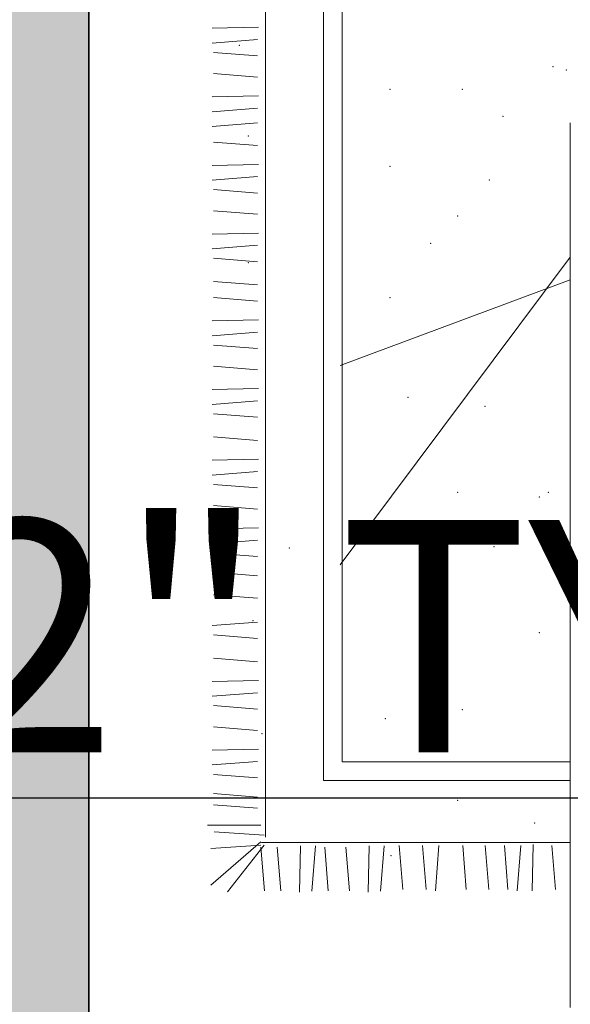
# Model space of a CAD drawing. Units: inches. Extents: x 1763 to 2368, y 1500 to 2097.
# Tile 18 of 24: x 2079 to 2109, y 1882 to 1935. Entities that reach past the tile are written whole.
import ezdxf

# ---------------------------------------------------------------- set-up
doc = ezdxf.new("R2010")
doc.units = ezdxf.units.IN
for name, color, linetype, lineweight in [('A-ANNO-DIMS', 2, 'Continuous', 18), ('A-FURN', 8, 'Continuous', 18), ('A-WALL', 7, 'Continuous', 35), ('A-WALL-PATT', 7, 'Continuous', 13)]:
    doc.layers.add(name, color=color, linetype=linetype, lineweight=lineweight)
doc.styles.get("Standard").update_dxf_attribs({"font": 'arial.ttf'})
doc.dimstyles.new('ISO-25', dxfattribs={"dimtxt": 12.5, "dimasz": 2.5, "dimexe": 1.25, "dimexo": 0.625, "dimtad": 1, "dimdec": 0, "dimlunit": 4, "dimtxsty": 'Standard', "dimblk": 'ARCHTICK', "dimcen": 2.5, "dimclrd": 3, "dimclrt": 4, "dimadec": 0, "dimazin": 0, "dimtfac": 1, "dimtdec": 0, "dimtmove": 0, "dimatfit": 3, "dimfxl": 1, "dimarcsym": 0})

# ---------------------------------------------------------------- blocks, each defined once
blk = doc.blocks.new('A$C77DF40FE')
for p, q in [((2.0097, 0.5844), (0.5839, 0.5844)), ((1.2963, 0.2134), (0.8003, 0.5844)), ((0.8369, 0.5844), (0.975, 0.2134)), ((1.6139, 0.217), (1.6139, 0.5844)), ((1.6439, 0.187), (1.6439, 0.5844)), ((1.7439, 0.087), (1.7439, 0.5844)), ((1.8197, 0.5605), (1.7489, 0.5548)), ((1.8218, 0.5229), (1.7471, 0.5245)), ((1.8218, 0.499), (1.7487, 0.5048)), ((1.8197, 0.4839), (1.7489, 0.4783)), ((1.8197, 0.453), (1.7489, 0.4474)), ((1.8197, 0.4168), (1.7489, 0.4111)), ((1.8218, 0.3671), (1.7487, 0.3728)), ((1.8197, 0.352), (1.7489, 0.3463)), ((1.8197, 0.3146), (1.7489, 0.3089)), ((1.7492, 0.2844), (1.8223, 0.2787)), ((1.7492, 0.2606), (1.824, 0.2589)), ((1.7513, 0.223), (1.8221, 0.2286)), ((0.3112, 0.217), (1.6139, 0.217)), ((1.7513, 0.1888), (1.8221, 0.1944)), ((0.3112, 0.187), (1.6439, 0.187)), ((1.7492, 0.1737), (1.8223, 0.1679)), ((1.7492, 0.1499), (1.824, 0.1482)), ((1.7513, 0.1122), (1.8221, 0.1179)), ((0.3112, 0.0935), (1.0155, 0.0935)), ((0.4313, 0.0075), (0.4296, 0.0823)), ((0.4551, 0.0075), (0.4493, 0.0806)), ((0.4702, 0.0096), (0.4758, 0.0804)), ((0.5043, 0.0096), (0.51, 0.0804)), ((0.542, 0.0075), (0.5403, 0.0823)), ((0.5658, 0.0075), (0.56, 0.0806)), ((0.5896, 0.0075), (0.5838, 0.0806)), ((0.6147, 0.0096), (0.6204, 0.0804)), ((0.6523, 0.0075), (0.6507, 0.0823)), ((0.6762, 0.0075), (0.6704, 0.0806)), ((0.6912, 0.0096), (0.6969, 0.0804)), ((0.7254, 0.0096), (0.7311, 0.0804)), ((0.7631, 0.0075), (0.7614, 0.0823)), ((0.7869, 0.0075), (0.7811, 0.0806)), ((0.802, 0.0096), (0.8076, 0.0804)), ((0.8394, 0.0096), (0.8451, 0.0804)), ((0.8654, 0.0096), (0.8711, 0.0804)), ((0.9031, 0.0075), (0.9014, 0.0823)), ((0.9269, 0.0075), (0.9212, 0.0806)), ((0.942, 0.0096), (0.9477, 0.0804)), ((0.9762, 0.0096), (0.9818, 0.0804)), ((1.0138, 0.0075), (1.0122, 0.0823)), ((1.0155, 0.0935), (1.7355, 0.0935)), ((1.0376, 0.0075), (1.0319, 0.0806)), ((1.0527, 0.0096), (1.0584, 0.0804)), ((1.0901, 0.0096), (1.0958, 0.0804)), ((1.1278, 0.0075), (1.1261, 0.0823)), ((1.1516, 0.0075), (1.1459, 0.0806)), ((1.1667, 0.0096), (1.1724, 0.0804)), ((1.2009, 0.0096), (1.2065, 0.0804)), ((1.2385, 0.0075), (1.2368, 0.0823)), ((1.2623, 0.0075), (1.2566, 0.0806)), ((1.2774, 0.0096), (1.2831, 0.0804)), ((1.3083, 0.0096), (1.314, 0.0804)), ((1.3446, 0.0096), (1.3503, 0.0804)), ((1.3943, 0.0075), (1.3885, 0.0806)), ((1.4094, 0.0096), (1.415, 0.0804)), ((1.4468, 0.0096), (1.4525, 0.0804)), ((1.4844, 0.0075), (1.4828, 0.0823)), ((1.5083, 0.0075), (1.5025, 0.0806)), ((1.5233, 0.0096), (1.529, 0.0804)), ((1.5575, 0.0096), (1.5632, 0.0804)), ((1.5951, 0.0075), (1.5935, 0.0823)), ((1.619, 0.0075), (1.6132, 0.0806)), ((1.6341, 0.0096), (1.6397, 0.0804)), ((1.665, 0.0096), (1.6706, 0.0804)), ((1.6831, 0.0096), (1.6888, 0.0804)), ((1.7162, 0.0857), (1.7162, 0)), ((1.7323, 0.0911), (1.7269, 0.0107)), ((1.743, 0.0857), (1.8126, 0.0054)), ((1.7483, 0.0911), (1.8233, 0.0322)), ((1.7483, 0.0857), (1.7537, 0.0054)), ((1.7513, 0.0858), (1.8221, 0.0915))]:
    blk.add_line(p, q)
for p in [(0.4984, 0.5782), (1.3453, 0.5782), (0.4931, 0.5564), (1.1794, 0.5491), (1.1867, 0.5345), (1.4058, 0.5345), (1.7124, 0.5272), (0.5734, 0.4761), (1.2671, 0.4615), (0.6757, 0.4542), (1.0407, 0.4469), (0.5296, 0.4104), (0.7341, 0.4032), (1.1794, 0.4032), (1.5299, 0.4104), (1.6759, 0.4032), (1.4788, 0.3813), (0.7779, 0.3594), (1.2963, 0.3448), (1.4204, 0.3448), (1.0261, 0.3229), (0.5296, 0.2937), (0.6538, 0.2937), (0.8655, 0.2937), (1.5445, 0.2864), (1.7652, 0.2958), (1.2693, 0.1315), (1.5686, 0.0878), (0.6049, 0.0659), (0.8093, 0.0659), (1.3861, 0.0732), (0.4588, 0.0513)]:
    blk.add_point(p)
blk = doc.blocks.new('_ArchTick')
at = {"color": 0, "linetype": 'ByBlock', "const_width": 0.15}
blk.add_lwpolyline([(-0.5, -0.5), (0.5, 0.5)], dxfattribs=at)
blk = doc.blocks.new('*D23')
at = {"layer": 'A-ANNO-DIMS', "color": 0, "lineweight": -2, "transparency": 16777216}
for p, q in [((2089.477, 1949.977), (2089.477, 1963.985)), ((2178.698, 1949.977), (2178.698, 1963.985))]:
    blk.add_line(p, q, dxfattribs=at)
at = {"layer": 'A-ANNO-DIMS', "color": 3, "lineweight": -2, "transparency": 16777216}
for p, q in [((2089.477, 1962.735), (2178.698, 1962.735)), ((2178.698, 1962.735), (2367.732, 1962.735))]:
    blk.add_line(p, q, dxfattribs=at)
at = {"layer": 'Defpoints', "color": 0, "transparency": 16777216}
for p in [(2178.698, 1962.735), (2089.477, 1949.352), (2178.698, 1949.352)]:
    blk.add_point(p, dxfattribs=at)
at = {"layer": 'A-ANNO-DIMS', "color": 3, "lineweight": -2, "transparency": 16777216, "xscale": 2.5, "yscale": 2.5, "zscale": 2.5, "rotation": 180}
blk.add_blockref('_ArchTick', (2089.477, 1962.735), dxfattribs=at)
at = {"layer": 'A-ANNO-DIMS', "color": 3, "lineweight": -2, "transparency": 16777216, "xscale": 2.5, "yscale": 2.5, "zscale": 2.5}
blk.add_blockref('_ArchTick', (2178.698, 1962.735), dxfattribs=at)
at = {"layer": 'A-ANNO-DIMS', "color": 4, "transparency": 16777216, "insert": (2274.465, 1969.828), "char_height": 12.5, "attachment_point": 5}
blk.add_mtext('BED GROUP 7\'-5" TYP.', dxfattribs=at)
blk = doc.blocks.new('*D34')
at = {"layer": 'A-ANNO-DIMS', "color": 0, "lineweight": -2, "transparency": 16777216}
for p, q in [((2001.644, 1895.481), (2001.644, 1892.281)), ((2013.092, 1895.481), (2013.092, 1892.281))]:
    blk.add_line(p, q, dxfattribs=at)
at = {"layer": 'A-ANNO-DIMS', "color": 3, "lineweight": -2, "transparency": 16777216}
for p, q in [((2001.644, 1893.531), (2013.092, 1893.531)), ((2013.092, 1893.531), (2131.874, 1893.531))]:
    blk.add_line(p, q, dxfattribs=at)
at = {"layer": 'Defpoints', "color": 0, "transparency": 16777216}
for p in [(2001.644, 1896.106), (2013.092, 1896.106), (2013.092, 1893.531)]:
    blk.add_point(p, dxfattribs=at)
at = {"layer": 'A-ANNO-DIMS', "color": 3, "lineweight": -2, "transparency": 16777216, "xscale": 2.5, "yscale": 2.5, "zscale": 2.5, "rotation": 180}
blk.add_blockref('_ArchTick', (2001.644, 1893.531), dxfattribs=at)
at = {"layer": 'A-ANNO-DIMS', "color": 3, "lineweight": -2, "transparency": 16777216, "xscale": 2.5, "yscale": 2.5, "zscale": 2.5}
blk.add_blockref('_ArchTick', (2013.092, 1893.531), dxfattribs=at)
at = {"layer": 'A-ANNO-DIMS', "color": 4, "transparency": 16777216, "insert": (2073.733, 1900.619), "char_height": 12.5, "attachment_point": 5}
blk.add_mtext('0\'-11 1/2" TYP.', dxfattribs=at)
blk = doc.blocks.new('*D62')
at = {"layer": 'A-ANNO-DIMS', "color": 0, "lineweight": -2, "transparency": 16777216}
for p, q in [((2083.092, 1980.648), (2083.092, 1509.906)), ((2120.612, 1980.648), (2120.612, 1509.906))]:
    blk.add_line(p, q, dxfattribs=at)
at = {"layer": 'A-ANNO-DIMS', "color": 3, "lineweight": -2, "transparency": 16777216}
for p, q in [((2083.092, 1511.156), (2120.612, 1511.156)), ((2120.612, 1511.156), (2186.709, 1511.156))]:
    blk.add_line(p, q, dxfattribs=at)
at = {"layer": 'Defpoints', "color": 0, "transparency": 16777216}
for p in [(2083.092, 1981.273), (2120.612, 1981.273), (2120.612, 1511.156)]:
    blk.add_point(p, dxfattribs=at)
at = {"layer": 'A-ANNO-DIMS', "color": 3, "lineweight": -2, "transparency": 16777216, "xscale": 2.5, "yscale": 2.5, "zscale": 2.5, "rotation": 180}
blk.add_blockref('_ArchTick', (2083.092, 1511.156), dxfattribs=at)
at = {"layer": 'A-ANNO-DIMS', "color": 3, "lineweight": -2, "transparency": 16777216, "xscale": 2.5, "yscale": 2.5, "zscale": 2.5}
blk.add_blockref('_ArchTick', (2120.612, 1511.156), dxfattribs=at)
at = {"layer": 'A-ANNO-DIMS', "color": 4, "transparency": 16777216, "insert": (2154.91, 1518.249), "char_height": 12.5, "attachment_point": 5}
blk.add_mtext('3\'-1 1/2"', dxfattribs=at)
blk = doc.blocks.new('*D72')
at = {"layer": 'A-ANNO-DIMS', "color": 0, "lineweight": -2, "transparency": 16777216}
for p, q in [((2018.092, 1885.898), (2018.092, 2072.023)), ((2049.737, 1885.898), (2049.737, 2072.023))]:
    blk.add_line(p, q, dxfattribs=at)
at = {"layer": 'A-ANNO-DIMS', "color": 3, "lineweight": -2, "transparency": 16777216}
for p, q in [((2018.092, 2070.773), (2049.737, 2070.773)), ((2049.737, 2070.773), (2116.055, 2070.773))]:
    blk.add_line(p, q, dxfattribs=at)
at = {"layer": 'Defpoints', "color": 0, "transparency": 16777216}
for p in [(2049.737, 2070.773), (2018.092, 1885.273), (2049.737, 1885.273)]:
    blk.add_point(p, dxfattribs=at)
at = {"layer": 'A-ANNO-DIMS', "color": 3, "lineweight": -2, "transparency": 16777216, "xscale": 2.5, "yscale": 2.5, "zscale": 2.5, "rotation": 180}
blk.add_blockref('_ArchTick', (2018.092, 2070.773), dxfattribs=at)
at = {"layer": 'A-ANNO-DIMS', "color": 3, "lineweight": -2, "transparency": 16777216, "xscale": 2.5, "yscale": 2.5, "zscale": 2.5}
blk.add_blockref('_ArchTick', (2049.737, 2070.773), dxfattribs=at)
at = {"layer": 'A-ANNO-DIMS', "color": 4, "transparency": 16777216, "insert": (2084.146, 2077.861), "char_height": 12.5, "attachment_point": 5}
blk.add_mtext('2\'-7 1/2"', dxfattribs=at)
blk = doc.blocks.new('*D78')
at = {"layer": 'A-ANNO-DIMS', "color": 0, "lineweight": -2, "transparency": 16777216}
for p, q in [((1996.717, 1981.273), (2217.842, 1981.273)), ((1986.217, 1948.273), (2217.842, 1948.273))]:
    blk.add_line(p, q, dxfattribs=at)
at = {"layer": 'A-ANNO-DIMS', "color": 3, "lineweight": -2, "transparency": 16777216}
for p, q in [((2216.592, 1981.273), (2216.592, 1948.273)), ((2216.592, 1948.273), (2216.592, 1911.081))]:
    blk.add_line(p, q, dxfattribs=at)
at = {"layer": 'Defpoints', "color": 0, "transparency": 16777216}
for p in [(1996.092, 1981.273), (1985.592, 1948.273), (2216.592, 1948.273)]:
    blk.add_point(p, dxfattribs=at)
at = {"layer": 'A-ANNO-DIMS', "color": 3, "lineweight": -2, "transparency": 16777216, "xscale": 2.5, "yscale": 2.5, "zscale": 2.5}
for p, rotation in [((2216.592, 1981.273), 90), ((2216.592, 1948.273), 270)]:
    blk.add_blockref('_ArchTick', p, dxfattribs=dict(at, rotation=rotation))
at = {"layer": 'A-ANNO-DIMS', "color": 4, "transparency": 16777216, "insert": (2209.585, 1928.427), "char_height": 12.5, "attachment_point": 5, "rotation": 90}
blk.add_mtext('2\'-9"', dxfattribs=at)

msp = doc.modelspace()

# ---------------------------------------------------------------- hatches: boundary and pattern name
at = {"layer": 'A-WALL-PATT'}
h = msp.add_hatch(color=256, dxfattribs=at)
h.dxf.hatch_style = 1
h.paths.add_polyline_path([(1838.092, 2034.273), (1838.092, 2043.273), (1829.092, 2043.273), (1829.092, 1953.387), (1838.092, 1953.387)])
h.paths.add_polyline_path([(1838.092, 1913.101), (1829.092, 1913.101), (1829.092, 1862.202), (1838.092, 1862.202)])
h.paths.add_polyline_path([(1838.092, 1825.59), (1829.092, 1825.59), (1829.092, 1738.643), (1838.092, 1738.643)])
h.paths.add_polyline_path([(1895.592, 1885.273), (1838.092, 1885.273), (1838.092, 1880.273), (1895.592, 1880.273)])
h.paths.add_polyline_path([(1857.389, 1784.273), (1838.092, 1784.273), (1838.092, 1779.273), (1857.389, 1779.273)])
h.paths.add_polyline_path([(1958.092, 1981.273), (1971.455, 1981.273), (1971.455, 1986.273), (1968.568, 1986.273), (1958.092, 1986.273), (1953.092, 1986.273), (1927.39, 1986.273), (1927.39, 1981.273), (1953.092, 1981.273), (1953.092, 1885.273), (1932.014, 1885.273), (1932.014, 1880.273), (1959.134, 1880.273), (1959.134, 1883.738), (1959.134, 1885.273), (1958.092, 1885.273)])
h.paths.add_polyline_path([(2018.092, 1981.273), (2031.019, 1981.273), (2031.019, 1986.273), (2018.092, 1986.273), (2013.092, 1986.273), (2001.233, 1986.273), (2001.233, 1981.273), (2013.092, 1981.273), (2013.092, 1885.273), (1982.182, 1885.273, -0.016629), (1982.233, 1883.738), (1982.233, 1880.273), (2049.686, 1880.273), (2049.686, 1883.738, -0.016629), (2049.737, 1885.273), (2018.092, 1885.273)])
h.paths.add_polyline_path([(2083.092, 1981.273), (2120.612, 1981.273), (2120.612, 1986.273), (2083.092, 1986.273), (2078.092, 1986.273), (2063.143, 1986.273), (2063.143, 1981.273), (2078.092, 1981.273), (2078.092, 1885.273), (2072.785, 1885.273), (2072.785, 1883.738), (2072.785, 1880.273), (2078.092, 1880.273), (2078.092, 1866.867), (2081.557, 1866.867, -0.016629), (2083.092, 1866.816)])
h.paths.add_polyline_path([(1871.675, 1635.273), (1838.092, 1635.273), (1838.092, 1626.273), (1871.675, 1626.273)], flags=17)
h.paths.add_polyline_path([(2100.577, 1688.273), (2060.092, 1688.273), (2060.092, 1679.273), (2100.577, 1679.273)], flags=17)
h.paths.add_polyline_path([(2180.092, 1688.273), (2148.744, 1688.273), (2148.744, 1679.273), (2180.092, 1679.273)], flags=17)
h.paths.add_polyline_path([(2189.092, 1746.219), (2180.092, 1746.219), (2180.092, 1743.417), (2180.123, 1743.417), (2180.123, 1726.723), (2180.092, 1572.273), (2034.907, 1572.273), (2034.907, 1565.601), (2034.907, 1563.273), (2189.092, 1563.273)])
h.paths.add_polyline_path([(2060.092, 1802.347, -0.016629), (2058.557, 1802.296), (2055.092, 1802.296), (2055.092, 1635.273), (2042.484, 1635.273), (2042.484, 1629.738), (2042.484, 1626.273), (2055.092, 1626.273), (2055.092, 1599.273), (2040.269, 1599.273), (2040.269, 1590.273), (2060.092, 1590.273)])
h.paths.add_polyline_path([(2019.385, 1629.738, -0.060569), (2020.058, 1635.273), (1995.092, 1635.273), (1990.092, 1635.273), (1927.075, 1635.273), (1927.075, 1626.273), (1990.092, 1626.273), (1990.092, 1590.273), (1995.092, 1590.273), (2005.195, 1590.273), (2005.195, 1599.273), (1995.092, 1599.273), (1995.092, 1626.273), (2019.385, 1626.273)])
edge = h.paths.add_edge_path()
edge.add_line((2180.092, 1837.273), (2167.198, 1837.273))
edge.add_spline(control_points=[(2167.198, 1837.273), (2167.191, 1837.271), (2167.183, 1837.271), (2167.176, 1837.273)], knot_values=[168.955493, 168.955493, 168.955493, 168.955493, 169.065871, 169.065871, 169.065871, 169.065871], degree=3, periodic=0)
edge.add_spline(control_points=[(2167.176, 1837.273), (2166.556, 1837.377), (2166.326, 1846.161), (2165.708, 1846.244)], knot_values=[159.864705, 159.864705, 159.864705, 159.864705, 168.955493, 168.955493, 168.955493, 168.955493], degree=3, periodic=0)
edge.add_line((2167.122, 1837.273), (2163.16, 1837.273))
edge.add_spline(control_points=[(2163.16, 1837.273), (2163.158, 1837.273), (2163.156, 1837.273), (2163.155, 1837.273)], knot_values=[150.537172, 150.537172, 150.537172, 150.537172, 150.553797, 150.553797, 150.553797, 150.553797], degree=3, periodic=0)
edge.add_spline(control_points=[(2163.155, 1837.273), (2162.29, 1837.289), (2161.594, 1846.232), (2160.878, 1846.244)], knot_values=[141.293426, 141.293426, 141.293426, 141.293426, 150.537172, 150.537172, 150.537172, 150.537172], degree=3, periodic=0)
edge.add_line((2163.075, 1837.273), (2158.7, 1837.273))
edge.add_spline(control_points=[(2158.7, 1837.273), (2158.698, 1837.273), (2158.697, 1837.273), (2158.696, 1837.273)], knot_values=[132.033544, 132.033544, 132.033544, 132.033544, 132.049151, 132.049151, 132.049151, 132.049151], degree=3, periodic=0)
edge.add_spline(control_points=[(2158.696, 1837.273), (2157.972, 1837.288), (2157.262, 1846.233), (2156.393, 1846.244)], knot_values=[122.786021, 122.786021, 122.786021, 122.786021, 132.033544, 132.033544, 132.033544, 132.033544], degree=3, periodic=0)
edge.add_line((2158.629, 1837.273), (2153.839, 1837.273))
edge.add_spline(control_points=[(2153.839, 1837.273), (2153.831, 1837.271), (2153.823, 1837.271), (2153.816, 1837.273)], knot_values=[113.451585, 113.451585, 113.451585, 113.451585, 113.562103, 113.562103, 113.562103, 113.562103], degree=3, periodic=0)
edge.add_spline(control_points=[(2153.816, 1837.273), (2153.17, 1837.378), (2152.878, 1846.191), (2152.404, 1846.244)], knot_values=[0, 0, 0, 0, 9.081854, 9.081854, 9.081854, 9.081854], degree=3, periodic=0)
edge.add_line((2153.76, 1837.273), (2150.391, 1837.273))
edge.add_spline(control_points=[(2150.391, 1837.273), (2150.381, 1837.272), (2150.371, 1837.272), (2150.361, 1837.273)], knot_values=[95.069382, 95.069382, 95.069382, 95.069382, 95.17519, 95.17519, 95.17519, 95.17519], degree=3, periodic=0)
edge.add_spline(control_points=[(2150.361, 1837.273), (2149.487, 1837.373), (2148.419, 1846.194), (2147.589, 1846.244)], knot_values=[85.824599, 85.824599, 85.824599, 85.824599, 95.069382, 95.069382, 95.069382, 95.069382], degree=3, periodic=0)
edge.add_line((2150.286, 1837.273), (2145.43, 1837.273))
edge.add_spline(control_points=[(2145.43, 1837.273), (2145.426, 1837.273), (2145.423, 1837.273), (2145.419, 1837.273)], knot_values=[76.505559, 76.505559, 76.505559, 76.505559, 76.547811, 76.547811, 76.547811, 76.547811], degree=3, periodic=0)
edge.add_spline(control_points=[(2145.419, 1837.273), (2144.684, 1837.313), (2143.804, 1846.194), (2142.948, 1846.244)], knot_values=[67.23945, 67.23945, 67.23945, 67.23945, 76.505559, 76.505559, 76.505559, 76.505559], degree=3, periodic=0)
edge.add_line((2145.353, 1837.273), (2134.57, 1837.273))
edge.add_spline(control_points=[(2134.57, 1837.273), (2134.567, 1837.272), (2134.563, 1837.272), (2134.56, 1837.273)], knot_values=[39.001463, 39.001463, 39.001463, 39.001463, 39.045107, 39.045107, 39.045107, 39.045107], degree=3, periodic=0)
edge.add_spline(control_points=[(2134.56, 1837.273), (2133.872, 1837.313), (2133.397, 1845.853), (2132.328, 1846.244)], knot_values=[29.79778, 29.79778, 29.79778, 29.79778, 39.001463, 39.001463, 39.001463, 39.001463], degree=3, periodic=0)
edge.add_line((2134.498, 1837.273), (2128.075, 1837.273))
edge.add_spline(control_points=[(2128.075, 1837.273), (2128.026, 1837.26), (2127.978, 1837.26), (2127.931, 1837.273)], knot_values=[19.482067, 19.482067, 19.482067, 19.482067, 19.869396, 19.869396, 19.869396, 19.869396], degree=3, periodic=0)
edge.add_spline(control_points=[(2125.013, 1846.244), (2126.165, 1844.663), (2126.821, 1837.57), (2127.931, 1837.273)], knot_values=[10.389805, 10.389805, 10.389805, 10.389805, 19.482067, 19.482067, 19.482067, 19.482067], degree=3, periodic=0)
edge.add_line((2127.931, 1837.273), (2083.092, 1837.273))
edge.add_line((2083.092, 1837.273), (2083.092, 1843.768))
edge.add_line((2083.092, 1843.768), (2081.557, 1843.768))
edge.add_line((2081.557, 1843.768), (2078.092, 1843.768))
edge.add_line((2078.092, 1843.768), (2078.092, 1837.273))
edge.add_line((2078.092, 1837.273), (2055.092, 1837.273))
edge.add_line((2055.092, 1837.273), (2055.092, 1825.395))
edge.add_line((2055.092, 1825.395), (2058.557, 1825.395))
edge.add_line((2058.557, 1825.395), (2060.092, 1825.395))
edge.add_line((2060.092, 1825.395), (2060.092, 1832.273))
edge.add_line((2060.092, 1832.273), (2122.437, 1832.273))
edge.add_spline(control_points=[(2122.437, 1832.273), (2122.727, 1832.584), (2123.008, 1832.617), (2123.275, 1832.273)], knot_values=[5.972033, 5.972033, 5.972033, 5.972033, 8.057258, 8.057258, 8.057258, 8.057258], degree=3, periodic=0)
edge.add_line((2123.275, 1832.273), (2137.951, 1832.273))
edge.add_spline(control_points=[(2137.951, 1832.273), (2137.961, 1832.274), (2137.971, 1832.274), (2137.98, 1832.273)], knot_values=[53.926862, 53.926862, 53.926862, 53.926862, 54.030075, 54.030075, 54.030075, 54.030075], degree=3, periodic=0)
edge.add_spline(control_points=[(2139.716, 1825.016), (2139.281, 1825.062), (2138.671, 1832.176), (2137.98, 1832.273)], knot_values=[54.030075, 54.030075, 54.030075, 54.030075, 61.445194, 61.445194, 61.445194, 61.445194], degree=3, periodic=0)
edge.add_line((2138.045, 1832.273), (2140.962, 1832.273))
edge.add_spline(control_points=[(2140.962, 1832.273), (2140.971, 1832.274), (2140.98, 1832.274), (2140.988, 1832.273)], knot_values=[68.854182, 68.854182, 68.854182, 68.854182, 68.971237, 68.971237, 68.971237, 68.971237], degree=3, periodic=0)
edge.add_spline(control_points=[(2143.19, 1825.016), (2142.436, 1825.065), (2141.561, 1832.162), (2140.988, 1832.273)], knot_values=[68.971237, 68.971237, 68.971237, 68.971237, 76.444911, 76.444911, 76.444911, 76.444911], degree=3, periodic=0)
edge.add_line((2141.041, 1832.273), (2145.43, 1832.273))
edge.add_spline(control_points=[(2145.43, 1832.273), (2145.439, 1832.274), (2145.448, 1832.274), (2145.458, 1832.273)], knot_values=[84.039047, 84.039047, 84.039047, 84.039047, 84.124041, 84.124041, 84.124041, 84.124041], degree=3, periodic=0)
edge.add_spline(control_points=[(2148.108, 1825.016), (2147.34, 1825.02), (2146.303, 1832.193), (2145.458, 1832.273)], knot_values=[84.124041, 84.124041, 84.124041, 84.124041, 91.773891, 91.773891, 91.773891, 91.773891], degree=3, periodic=0)
edge.add_line((2145.538, 1832.273), (2150.393, 1832.273))
edge.add_spline(control_points=[(2150.393, 1832.273), (2150.419, 1832.277), (2150.445, 1832.277), (2150.472, 1832.273)], knot_values=[99.381577, 99.381577, 99.381577, 99.381577, 99.573457, 99.573457, 99.573457, 99.573457], degree=3, periodic=0)
edge.add_spline(control_points=[(2153.974, 1825.016), (2153.093, 1825.281), (2151.529, 1832.103), (2150.472, 1832.273)], knot_values=[99.573457, 99.573457, 99.573457, 99.573457, 107.218357, 107.218357, 107.218357, 107.218357], degree=3, periodic=0)
edge.add_line((2150.568, 1832.273), (2155.598, 1832.273))
edge.add_spline(control_points=[(2155.598, 1832.273), (2155.605, 1832.273), (2155.611, 1832.273), (2155.618, 1832.273)], knot_values=[114.933058, 114.933058, 114.933058, 114.933058, 115.013624, 115.013624, 115.013624, 115.013624], degree=3, periodic=0)
edge.add_spline(control_points=[(2158.285, 1825.016), (2157.395, 1825.074), (2156.252, 1832.197), (2155.618, 1832.273)], knot_values=[115.013624, 115.013624, 115.013624, 115.013624, 122.616269, 122.616269, 122.616269, 122.616269], degree=3, periodic=0)
edge.add_line((2155.678, 1832.273), (2165.195, 1832.273))
edge.add_spline(control_points=[(2165.195, 1832.273), (2165.198, 1832.273), (2165.201, 1832.273), (2165.204, 1832.273)], knot_values=[145.488477, 145.488477, 145.488477, 145.488477, 145.516379, 145.516379, 145.516379, 145.516379], degree=3, periodic=0)
edge.add_spline(control_points=[(2167.446, 1825.016), (2166.961, 1825.022), (2166.056, 1832.246), (2165.204, 1832.273)], knot_values=[145.516379, 145.516379, 145.516379, 145.516379, 153.105469, 153.105469, 153.105469, 153.105469], degree=3, periodic=0)
edge.add_line((2165.29, 1832.273), (2168.928, 1832.273))
edge.add_spline(control_points=[(2168.928, 1832.273), (2168.982, 1832.293), (2169.038, 1832.293), (2169.096, 1832.273)], knot_values=[160.517439, 160.517439, 160.517439, 160.517439, 160.939723, 160.939723, 160.939723, 160.939723], degree=3, periodic=0)
edge.add_spline(control_points=[(2171.086, 1828.645), (2170.355, 1830.369), (2169.624, 1832.094), (2169.096, 1832.273)], knot_values=[160.939723, 160.939723, 160.939723, 160.939723, 164.738835, 164.738835, 164.738835, 164.738835], degree=3, periodic=0)
edge.add_line((2169.096, 1832.273), (2180.092, 1832.273))
edge.add_line((2180.092, 1832.273), (2180.092, 1837.273))
h.paths.add_polyline_path([(2189.092, 1885.523), (2180.092, 1885.523), (2180.092, 1813.317), (2180.123, 1813.317), (2180.123, 1796.623), (2180.123, 1795.256), (2189.092, 1795.256)])
h.paths.add_polyline_path([(2180.092, 1986.273), (2166.28, 1986.273), (2166.28, 1981.273), (2180.092, 1981.273)])
h.paths.add_polyline_path([(2189.092, 2043.273), (2180.092, 2043.273), (2180.092, 2034.273), (2180.092, 1934.108), (2189.092, 1934.108)])
h.paths.add_polyline_path([(1838.092, 1681.592), (1829.092, 1681.592), (1829.092, 1563.273), (2003.864, 1563.273), (2003.864, 1565.601), (2003.864, 1572.273), (1838.092, 1572.273)])

# ---------------------------------------------------------------- linework, layer by layer
at = {"layer": 'A-WALL'}
msp.add_line((2083.092, 1866.816), (2083.092, 1981.273), dxfattribs=at)

# ---------------------------------------------------------------- block references
at = {"layer": 'A-FURN', "xscale": 33.38694677217886, "yscale": 33.38694677217886, "zscale": 33.38694677217886, "rotation": 270}
msp.add_blockref('A$C77DF40FE', (2089.477, 1949.352), dxfattribs=at)

# ---------------------------------------------------------------- dimensions: what is measured, and where the dimension line sits
at = {"layer": 'A-ANNO-DIMS'}
for base, p1, p2, picture, middle in [((2049.737, 2070.773), (2018.092, 1885.273), (2049.737, 1885.273), '*D72', (2084.146, 2077.861)), ((2120.612, 1511.156), (2083.092, 1981.273), (2120.612, 1981.273), '*D62', (2154.91, 1518.249))]:
    dim = msp.add_linear_dim(base=base, p1=p1, p2=p2, dimstyle='ISO-25', override={"dimdec": 1, "dimlfac": 1, "dimrnd": 0, "dimzin": 1, "dimdsep": 46, "dimlunit": 4, "dimfrac": 2}, dxfattribs=at)
    dim.commit()
    dim.dimension.update_dxf_attribs({"geometry": picture, "text_midpoint": middle})
for base, p1, p2, text, picture, middle in [((2178.698, 1962.735), (2089.477, 1949.352), (2178.698, 1949.352), 'BED GROUP <> TYP.', '*D23', (2274.465, 1969.828)), ((2013.092, 1893.531), (2001.644, 1896.106), (2013.092, 1896.106), '<> TYP.', '*D34', (2073.733, 1900.619))]:
    dim = msp.add_linear_dim(base=base, p1=p1, p2=p2, text=text, dimstyle='ISO-25', override={"dimdec": 1, "dimlfac": 1, "dimrnd": 0, "dimzin": 1, "dimdsep": 46, "dimlunit": 4, "dimfrac": 2}, dxfattribs=at)
    dim.commit()
    dim.dimension.update_dxf_attribs({"geometry": picture, "text_midpoint": middle})
dim = msp.add_linear_dim(base=(2216.592, 1948.273), p1=(1996.092, 1981.273), p2=(1985.592, 1948.273), angle=90, dimstyle='ISO-25', override={"dimdec": 1, "dimlfac": 1, "dimrnd": 0, "dimzin": 1, "dimdsep": 46, "dimlunit": 4, "dimfrac": 2}, dxfattribs=at)
dim.commit()
dim.dimension.update_dxf_attribs({"geometry": '*D78', "text_midpoint": (2209.585, 1928.427)})

doc.saveas('drawing.dxf')
